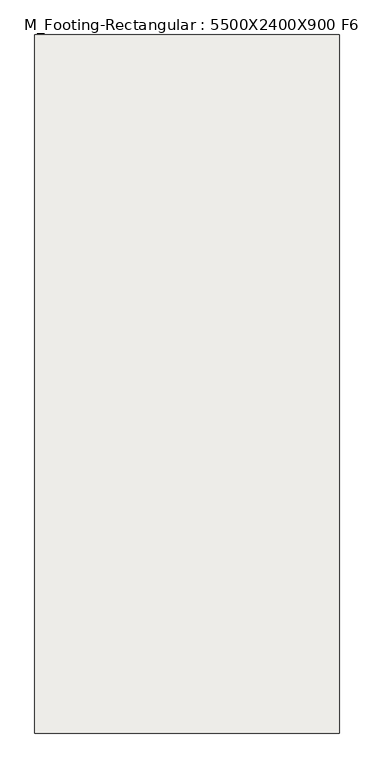
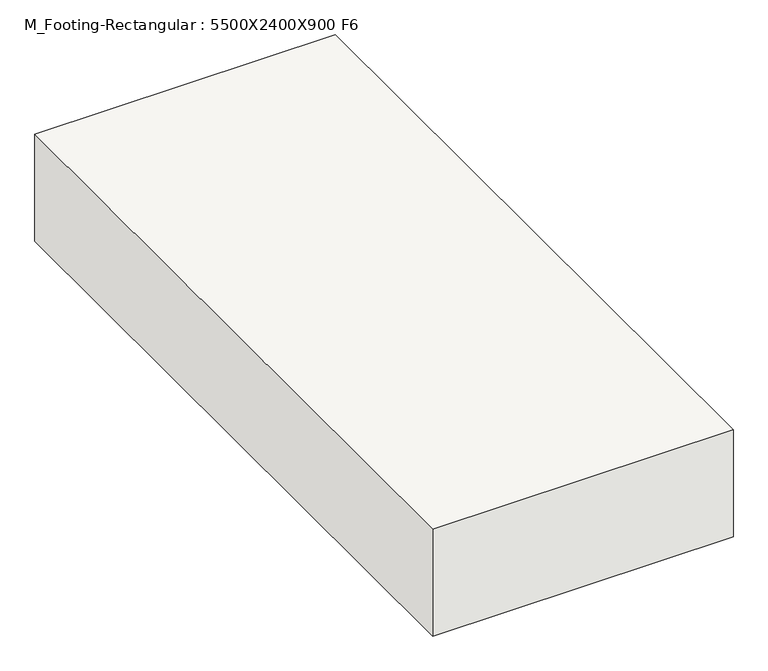
"""IFC4 building model written with IfcOpenShell, lengths in millimetres: slab geometry, M_Footing-Rectangular : 5500X2400X900 F6."""

from ifc_helpers import new_model, si_unit, frame, origin, place, context, project, spatial, polyline, outline, extrude, source, transform, mapped, element, save


def m_footing_rectangular_5500x2400x900_f6_6a8cdcd2(model_context):
    return source(origin(), model_context, "Body", "SweptSolid", [
        extrude(outline(polyline([(1200.0, 2750.0), (1200.0, -2750.0), (-1200.0, -2750.0), (-1200.0, 2750.0), (1200.0, 2750.0)])), frame((0.0, 0.0, -900.0), z_axis=(0.0, 0.0, 1.0), x_axis=(1.0, 0.0, 0.0)), (0.0, 0.0, 1.0), 900.0),
    ])


if __name__ == "__main__":
    model = new_model("IFC4")
    model_context = context("Model", 3, world=origin())
    ifc_project = project(units=[si_unit("LENGTHUNIT", "METRE", prefix="MILLI")], contexts=[model_context])
    site = spatial("IfcSite", under=ifc_project)
    building = spatial("IfcBuilding", under=site)
    placement = place(None, origin())
    m_footing_rectangular_5500x2400x900_f6_shape = m_footing_rectangular_5500x2400x900_f6_6a8cdcd2(model_context)
    element("IfcSlab", 1, ObjectType="M_Footing-Rectangular : 5500X2400X900 F6", at=placement, inside=building, context=model_context, shape_type="MappedRepresentation", body=[
        mapped(m_footing_rectangular_5500x2400x900_f6_shape, transform((0.0, 0.0, 0.0), x_axis=(1.0, 0.0, 0.0), y_axis=(0.0, 1.0, 0.0), z_axis=(0.0, 0.0, 1.0))),
    ])
    save(model, "model.ifc")

# Revit data of these elements
# Type "M_Footing-Rectangular : 5500X2400X900 F6"
#   Width = 2400 mm
#   Length = 5500 mm
#   Foundation Thickness = 900 mm
#   Structural Material [instance default] = Concrete, Cast-in-Place gray
#   Assembly Code = ""
# Element 1 (IfcSlab, "M_Footing-Rectangular : 5500X2400X900 F6")
#   Structural Material = Concrete, Cast In Situ
#   Materials on its faces: "Concrete, Cast In Situ"
# Materials
#   "Concrete, Cast-in-Place gray": class "Concrete", colour RGB 192 192 192, transparency 0, Description = "Cast-in-place concrete", Cost = 0
#   "Concrete, Cast In Situ": class "Concrete", colour RGB 192 192 192, transparency 0, Description = "physical material", Cost = 0
